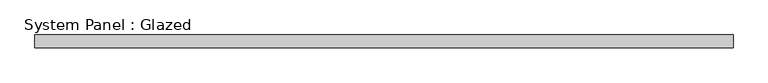
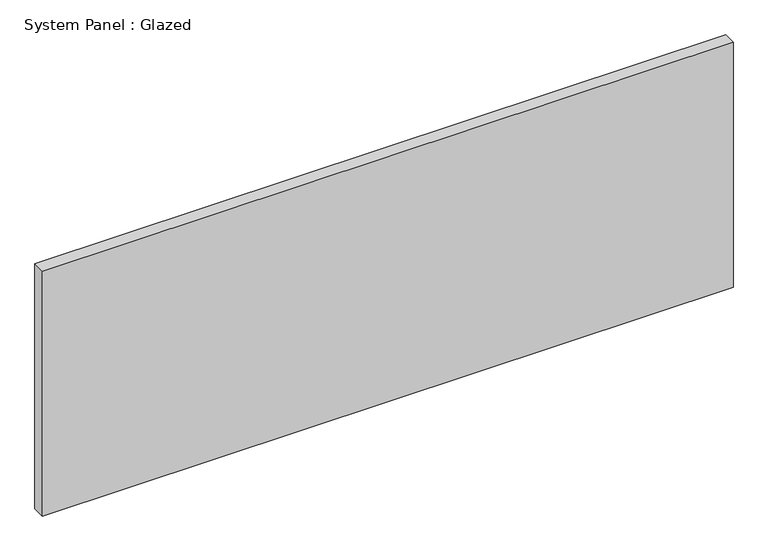
"""IFC4 building model written with IfcOpenShell, lengths in millimetres: plate geometry, System Panel : Glazed."""

from ifc_helpers import new_model, si_unit, origin, origin_with_axes, place, context, project, spatial, polyline, outline, extrude, source, transform, mapped, element, save


def system_panel_glazed_04da4e26(model_context):
    return source(origin(), model_context, "Body", "SweptSolid", [
        extrude(outline(polyline([(685.8000001, -44.45), (-685.8000001, -44.45), (-685.8000001, -19.05), (685.8000001, -19.05), (685.8000001, -44.45)])), origin_with_axes(), (0.0, 0.0, 1.0), 514.35),
    ])


if __name__ == "__main__":
    model = new_model("IFC4")
    model_context = context("Model", 3, world=origin())
    ifc_project = project(units=[si_unit("LENGTHUNIT", "METRE", prefix="MILLI")], contexts=[model_context])
    site = spatial("IfcSite", under=ifc_project)
    building = spatial("IfcBuilding", under=site)
    placement = place(None, origin())
    system_panel_glazed_shape = system_panel_glazed_04da4e26(model_context)
    element("IfcPlate", 1, ObjectType="System Panel : Glazed", at=placement, inside=building, context=model_context, shape_type="MappedRepresentation", body=[
        mapped(system_panel_glazed_shape, transform((0.0, 0.0, 0.0), x_axis=(1.0, 0.0, 0.0), y_axis=(0.0, 1.0, 0.0), z_axis=(0.0, 0.0, 1.0))),
    ])
    save(model, "model.ifc")

# Revit data of these elements
# Type "System Panel : Glazed"
#   Construction Type Id = "GSP4R"
#   Analytic Construction = "1/8 in Pilkington single glazing"
#   Visual Light Transmittance = 0.9
#   Solar Heat Gain Coefficient = 0.86
#   Heat Transfer Coefficient (U) = 1.18115 BTU/(h·ft²·°F)
#   Define Thermal Properties by = 1
# Element 1 (IfcPlate, "System Panel : Glazed")
#   Materials on its faces: "Glass"
# Materials
#   "Glass": class "Glass", colour RGB 0 128 192, transparency 0.75, Description = "Soda Lime Glass", Cost = 0
